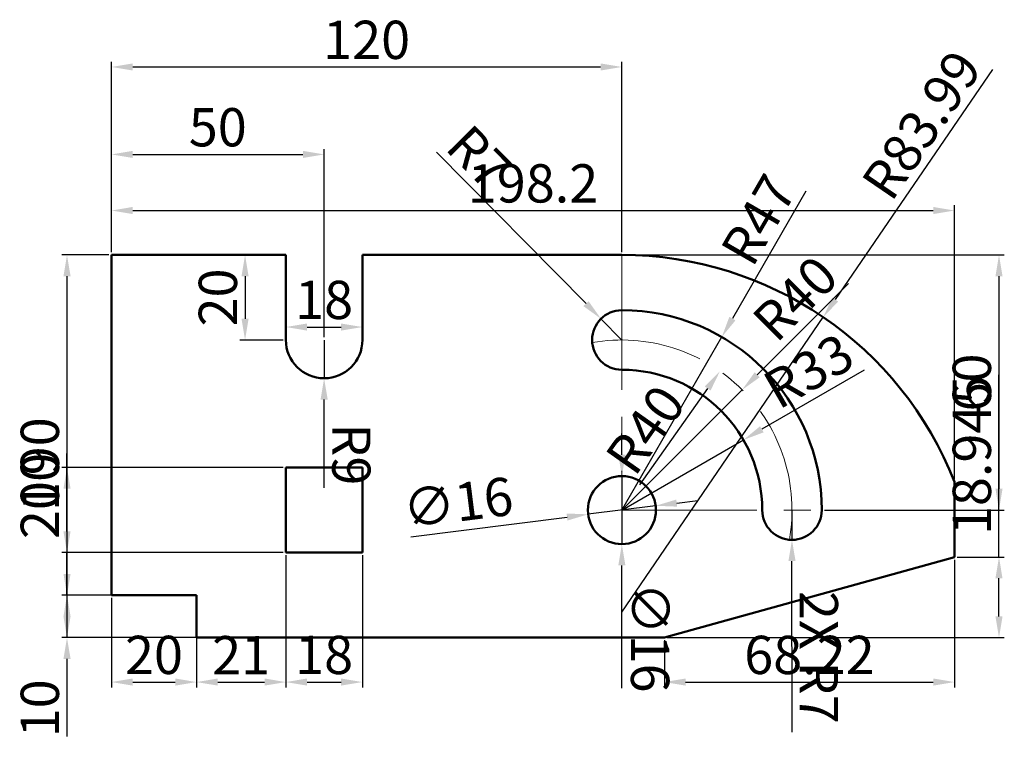
# Model space of a CAD drawing. Units: millimetres. Extents: x 2223 to 2454, y 1457 to 1626.
import ezdxf

# ---------------------------------------------------------------- set-up
doc = ezdxf.new("R2010")
doc.units = ezdxf.units.MM
doc.linetypes.add('CENTER', pattern=[50.8, 31.75, -6.35, 6.35, -6.35])
for name, color, linetype, lineweight in [('M-CNTR', 4, 'CENTER', 18), ('M-DIMS', 2, 'Continuous', 25), ('M-OUTL', 7, 'Continuous', 50)]:
    doc.layers.add(name, color=color, linetype=linetype, lineweight=lineweight)
doc.styles.get("Standard").update_dxf_attribs({"font": 'arial.ttf'})
doc.dimstyles.new('ISO-25', dxfattribs={"dimtxt": 9, "dimasz": 5, "dimexe": 1.25, "dimexo": 0.625, "dimtad": 1, "dimtxsty": 'Standard', "dimcen": 2.5, "dimadec": 0, "dimazin": 0, "dimtfac": 1, "dimtmove": 0, "dimatfit": 3, "dimfxl": 1, "dimarcsym": 0})

# ---------------------------------------------------------------- blocks, each defined once
blk = doc.blocks.new('*D1')
at = {"layer": 'Defpoints', "color": 0, "transparency": 16777216}
for p in [(2294.23, 1594.38), (2244.23, 1570.73), (2294.23, 1550.73)]:
    blk.add_point(p, dxfattribs=at)
at = {"layer": 'M-DIMS', "color": 0, "lineweight": -2, "transparency": 16777216}
for p, q in [((2244.23, 1571.36), (2244.23, 1595.63)), ((2294.23, 1551.36), (2294.23, 1595.63)), ((2249.23, 1594.38), (2289.23, 1594.38))]:
    blk.add_line(p, q, dxfattribs=at)
at = {"layer": 'M-DIMS', "color": 0, "transparency": 16777216}
for points in [[(2249.23, 1595.21), (2249.23, 1593.54), (2244.23, 1594.38)], [(2289.23, 1595.21), (2289.23, 1593.54), (2294.23, 1594.38)]]:
    blk.add_solid(points, dxfattribs=at)
at = {"layer": 'M-DIMS', "color": 0, "transparency": 16777216, "insert": (2269.23, 1599.6), "char_height": 9, "attachment_point": 5}
blk.add_mtext('50', dxfattribs=at)
blk = doc.blocks.new('*D2')
at = {"layer": 'Defpoints', "color": 0, "transparency": 16777216}
for p in [(2364.23, 1614.94), (2244.23, 1570.73), (2364.23, 1570.73)]:
    blk.add_point(p, dxfattribs=at)
at = {"layer": 'M-DIMS', "color": 0, "lineweight": -2, "transparency": 16777216}
for p, q in [((2244.23, 1571.36), (2244.23, 1616.19)), ((2364.23, 1571.36), (2364.23, 1616.19)), ((2249.23, 1614.94), (2359.23, 1614.94))]:
    blk.add_line(p, q, dxfattribs=at)
at = {"layer": 'M-DIMS', "color": 0, "transparency": 16777216}
for points in [[(2249.23, 1615.77), (2249.23, 1614.11), (2244.23, 1614.94)], [(2359.23, 1615.77), (2359.23, 1614.11), (2364.23, 1614.94)]]:
    blk.add_solid(points, dxfattribs=at)
at = {"layer": 'M-DIMS', "color": 0, "transparency": 16777216, "insert": (2304.23, 1620.16), "char_height": 9, "attachment_point": 5}
blk.add_mtext('120', dxfattribs=at)
blk = doc.blocks.new('*D3')
at = {"layer": 'Defpoints', "color": 0, "transparency": 16777216}
for p in [(2285.23, 1570.73), (2303.23, 1570.73), (2303.23, 1553.78)]:
    blk.add_point(p, dxfattribs=at)
at = {"layer": 'M-DIMS', "color": 0, "lineweight": -2, "transparency": 16777216}
for p, q in [((2285.23, 1570.11), (2285.23, 1552.53)), ((2303.23, 1570.11), (2303.23, 1552.53)), ((2290.23, 1553.78), (2298.23, 1553.78))]:
    blk.add_line(p, q, dxfattribs=at)
at = {"layer": 'M-DIMS', "color": 0, "transparency": 16777216}
for points in [[(2290.23, 1554.61), (2290.23, 1552.94), (2285.23, 1553.78)], [(2298.23, 1554.61), (2298.23, 1552.94), (2303.23, 1553.78)]]:
    blk.add_solid(points, dxfattribs=at)
at = {"layer": 'M-DIMS', "color": 0, "transparency": 16777216, "insert": (2294.23, 1559), "char_height": 9, "attachment_point": 5}
blk.add_mtext('18', dxfattribs=at)
blk = doc.blocks.new('*D4')
at = {"layer": 'Defpoints', "color": 0, "transparency": 16777216}
for p in [(2285.23, 1570.73), (2275.64, 1550.73), (2285.23, 1550.73)]:
    blk.add_point(p, dxfattribs=at)
at = {"layer": 'M-DIMS', "color": 0, "lineweight": -2, "transparency": 16777216}
for p, q in [((2284.61, 1570.73), (2274.39, 1570.73)), ((2275.64, 1565.73), (2275.64, 1555.73)), ((2284.61, 1550.73), (2274.39, 1550.73))]:
    blk.add_line(p, q, dxfattribs=at)
at = {"layer": 'M-DIMS', "color": 0, "transparency": 16777216}
for points in [[(2274.81, 1565.73), (2276.47, 1565.73), (2275.64, 1570.73)], [(2274.81, 1555.73), (2276.47, 1555.73), (2275.64, 1550.73)]]:
    blk.add_solid(points, dxfattribs=at)
at = {"layer": 'M-DIMS', "color": 0, "transparency": 16777216, "insert": (2270.42, 1560.73), "char_height": 9, "attachment_point": 5, "rotation": 90}
blk.add_mtext('20', dxfattribs=at)
blk = doc.blocks.new('*D5')
at = {"layer": 'Defpoints', "color": 0, "transparency": 16777216}
for p in [(2359.32, 1555.72), (2364.23, 1550.73)]:
    blk.add_point(p, dxfattribs=at)
at = {"layer": 'M-DIMS', "color": 0, "lineweight": -2, "transparency": 16777216}
for p, q in [((2320.69, 1594.87), (2355.81, 1559.28)), ((2364.23, 1550.73), (2359.32, 1555.72))]:
    blk.add_line(p, q, dxfattribs=at)
at = {"layer": 'M-DIMS', "color": 0, "transparency": 16777216}
blk.add_solid([(2356.4, 1559.86), (2355.21, 1558.69), (2359.32, 1555.72)], dxfattribs=at)
at = {"layer": 'M-DIMS', "color": 0, "transparency": 16777216, "insert": (2329.87, 1592.86), "char_height": 9, "attachment_point": 5, "rotation": 314.6114}
blk.add_mtext('R7', dxfattribs=at)
blk = doc.blocks.new('*D6')
at = {"layer": 'Defpoints', "color": 0, "transparency": 16777216}
for p in [(2387.3, 1543.42), (2364.23, 1510.73)]:
    blk.add_point(p, dxfattribs=at)
at = {"layer": 'M-DIMS', "color": 0, "lineweight": -2, "transparency": 16777216}
blk.add_line((2368.43, 1516.68), (2384.41, 1539.33), dxfattribs=at)
at = {"layer": 'M-DIMS', "color": 0, "transparency": 16777216}
blk.add_solid([(2383.73, 1539.81), (2385.09, 1538.85), (2387.3, 1543.42)], dxfattribs=at)
at = {"layer": 'M-DIMS', "color": 0, "transparency": 16777216, "insert": (2370.71, 1528.97), "char_height": 9, "attachment_point": 5, "rotation": 54.7921}
blk.add_mtext('R40', dxfattribs=at)
blk = doc.blocks.new('*D7')
at = {"layer": 'Defpoints', "color": 0, "transparency": 16777216}
for p in [(2372.17, 1511.74), (2356.3, 1509.73)]:
    blk.add_point(p, dxfattribs=at)
at = {"layer": 'M-DIMS', "color": 0, "lineweight": -2, "transparency": 16777216}
for p, q in [((2372.17, 1511.74), (2356.3, 1509.73)), ((2377.13, 1512.37), (2382.09, 1513)), ((2314.65, 1504.44), (2351.34, 1509.1))]:
    blk.add_line(p, q, dxfattribs=at)
at = {"layer": 'M-DIMS', "color": 0, "transparency": 16777216}
for points in [[(2377.03, 1513.2), (2377.24, 1511.54), (2372.17, 1511.74)], [(2351.23, 1509.92), (2351.44, 1508.27), (2356.3, 1509.73)]]:
    blk.add_solid(points, dxfattribs=at)
at = {"layer": 'M-DIMS', "color": 0, "transparency": 16777216, "insert": (2325.83, 1511.38), "char_height": 9, "attachment_point": 5, "rotation": 7.2276}
blk.add_mtext('∅16', dxfattribs=at)
blk = doc.blocks.new('*D8')
at = {"layer": 'Defpoints', "color": 0, "transparency": 16777216}
for p in [(2442.45, 1581.18), (2244.23, 1570.73), (2442.45, 1517.34)]:
    blk.add_point(p, dxfattribs=at)
at = {"layer": 'M-DIMS', "color": 0, "lineweight": -2, "transparency": 16777216}
for p, q in [((2244.23, 1571.36), (2244.23, 1582.43)), ((2249.23, 1581.18), (2437.45, 1581.18)), ((2442.45, 1517.97), (2442.45, 1582.43))]:
    blk.add_line(p, q, dxfattribs=at)
at = {"layer": 'M-DIMS', "color": 0, "transparency": 16777216}
for points in [[(2249.23, 1582.02), (2249.23, 1580.35), (2244.23, 1581.18)], [(2437.45, 1582.02), (2437.45, 1580.35), (2442.45, 1581.18)]]:
    blk.add_solid(points, dxfattribs=at)
at = {"layer": 'M-DIMS', "color": 0, "transparency": 16777216, "insert": (2343.34, 1586.4), "char_height": 9, "attachment_point": 5}
blk.add_mtext('198.2', dxfattribs=at)
blk = doc.blocks.new('*D9')
at = {"layer": 'Defpoints', "color": 0, "transparency": 16777216}
for p in [(2244.23, 1570.73), (2233.78, 1480.73), (2374.23, 1480.73)]:
    blk.add_point(p, dxfattribs=at)
at = {"layer": 'M-DIMS', "color": 0, "lineweight": -2, "transparency": 16777216}
for p, q in [((2243.61, 1570.73), (2232.53, 1570.73)), ((2233.78, 1565.73), (2233.78, 1485.73)), ((2373.61, 1480.73), (2232.53, 1480.73))]:
    blk.add_line(p, q, dxfattribs=at)
at = {"layer": 'M-DIMS', "color": 0, "transparency": 16777216}
for points in [[(2232.95, 1565.73), (2234.62, 1565.73), (2233.78, 1570.73)], [(2232.95, 1485.73), (2234.62, 1485.73), (2233.78, 1480.73)]]:
    blk.add_solid(points, dxfattribs=at)
at = {"layer": 'M-DIMS', "color": 0, "transparency": 16777216, "insert": (2228.56, 1525.73), "char_height": 9, "attachment_point": 5, "rotation": 90}
blk.add_mtext('90', dxfattribs=at)
blk = doc.blocks.new('*D10')
at = {"layer": 'Defpoints', "color": 0, "transparency": 16777216}
for p in [(2244.23, 1490.73), (2264.23, 1490.73), (2264.23, 1470.28)]:
    blk.add_point(p, dxfattribs=at)
at = {"layer": 'M-DIMS', "color": 0, "lineweight": -2, "transparency": 16777216}
for p, q in [((2244.23, 1490.11), (2244.23, 1469.03)), ((2264.23, 1490.11), (2264.23, 1469.03)), ((2249.23, 1470.28), (2259.23, 1470.28))]:
    blk.add_line(p, q, dxfattribs=at)
at = {"layer": 'M-DIMS', "color": 0, "transparency": 16777216}
for points in [[(2249.23, 1471.12), (2249.23, 1469.45), (2244.23, 1470.28)], [(2259.23, 1471.12), (2259.23, 1469.45), (2264.23, 1470.28)]]:
    blk.add_solid(points, dxfattribs=at)
at = {"layer": 'M-DIMS', "color": 0, "transparency": 16777216, "insert": (2254.23, 1475.5), "char_height": 9, "attachment_point": 5}
blk.add_mtext('20', dxfattribs=at)
blk = doc.blocks.new('*D11')
at = {"layer": 'Defpoints', "color": 0, "transparency": 16777216}
for p in [(2264.23, 1490.73), (2233.78, 1480.73), (2264.23, 1480.73)]:
    blk.add_point(p, dxfattribs=at)
at = {"layer": 'M-DIMS', "color": 0, "lineweight": -2, "transparency": 16777216}
for p, q in [((2233.78, 1495.73), (2233.78, 1500.73)), ((2263.61, 1490.73), (2232.53, 1490.73)), ((2233.78, 1490.73), (2233.78, 1480.73)), ((2263.61, 1480.73), (2232.53, 1480.73)), ((2233.78, 1475.73), (2233.78, 1457.47))]:
    blk.add_line(p, q, dxfattribs=at)
at = {"layer": 'M-DIMS', "color": 0, "transparency": 16777216}
for points in [[(2232.95, 1495.73), (2234.62, 1495.73), (2233.78, 1490.73)], [(2232.95, 1475.73), (2234.62, 1475.73), (2233.78, 1480.73)]]:
    blk.add_solid(points, dxfattribs=at)
at = {"layer": 'M-DIMS', "color": 0, "transparency": 16777216, "insert": (2228.56, 1464.1), "char_height": 9, "attachment_point": 5, "rotation": 90}
blk.add_mtext('10', dxfattribs=at)
blk = doc.blocks.new('*D12')
at = {"layer": 'Defpoints', "color": 0, "transparency": 16777216}
for p in [(2442.45, 1499.68), (2374.23, 1480.73), (2442.45, 1470.28)]:
    blk.add_point(p, dxfattribs=at)
at = {"layer": 'M-DIMS', "color": 0, "lineweight": -2, "transparency": 16777216}
for p, q in [((2442.45, 1499.05), (2442.45, 1469.03)), ((2374.23, 1480.11), (2374.23, 1469.03)), ((2379.23, 1470.28), (2437.45, 1470.28))]:
    blk.add_line(p, q, dxfattribs=at)
at = {"layer": 'M-DIMS', "color": 0, "transparency": 16777216}
for points in [[(2379.23, 1471.12), (2379.23, 1469.45), (2374.23, 1470.28)], [(2437.45, 1471.12), (2437.45, 1469.45), (2442.45, 1470.28)]]:
    blk.add_solid(points, dxfattribs=at)
at = {"layer": 'M-DIMS', "color": 0, "transparency": 16777216, "insert": (2408.34, 1475.5), "char_height": 9, "attachment_point": 5}
blk.add_mtext('68.22', dxfattribs=at)
blk = doc.blocks.new('*D13')
at = {"layer": 'Defpoints', "color": 0, "transparency": 16777216}
for p in [(2442.45, 1499.68), (2452.9, 1499.68), (2374.23, 1480.73)]:
    blk.add_point(p, dxfattribs=at)
at = {"layer": 'M-DIMS', "color": 0, "lineweight": -2, "transparency": 16777216}
for p, q in [((2452.9, 1499.68), (2452.9, 1542.51)), ((2443.08, 1499.68), (2454.15, 1499.68)), ((2452.9, 1485.73), (2452.9, 1494.68)), ((2374.86, 1480.73), (2454.15, 1480.73))]:
    blk.add_line(p, q, dxfattribs=at)
at = {"layer": 'M-DIMS', "color": 0, "transparency": 16777216}
for points in [[(2452.07, 1494.68), (2453.73, 1494.68), (2452.9, 1499.68)], [(2452.07, 1485.73), (2453.73, 1485.73), (2452.9, 1480.73)]]:
    blk.add_solid(points, dxfattribs=at)
at = {"layer": 'M-DIMS', "color": 0, "transparency": 16777216, "insert": (2447.68, 1523.6), "char_height": 9, "attachment_point": 5, "rotation": 90}
blk.add_mtext('18.945', dxfattribs=at)
blk = doc.blocks.new('*D14')
at = {"layer": 'Defpoints', "color": 0, "transparency": 16777216}
for p in [(2285.23, 1500.73), (2303.23, 1500.73), (2303.23, 1470.28)]:
    blk.add_point(p, dxfattribs=at)
at = {"layer": 'M-DIMS', "color": 0, "lineweight": -2, "transparency": 16777216}
for p, q in [((2285.23, 1500.11), (2285.23, 1469.03)), ((2303.23, 1500.11), (2303.23, 1469.03)), ((2290.23, 1470.28), (2298.23, 1470.28))]:
    blk.add_line(p, q, dxfattribs=at)
at = {"layer": 'M-DIMS', "color": 0, "transparency": 16777216}
for points in [[(2290.23, 1471.12), (2290.23, 1469.45), (2285.23, 1470.28)], [(2298.23, 1471.12), (2298.23, 1469.45), (2303.23, 1470.28)]]:
    blk.add_solid(points, dxfattribs=at)
at = {"layer": 'M-DIMS', "color": 0, "transparency": 16777216, "insert": (2294.23, 1475.5), "char_height": 9, "attachment_point": 5}
blk.add_mtext('18', dxfattribs=at)
blk = doc.blocks.new('*D15')
at = {"layer": 'Defpoints', "color": 0, "transparency": 16777216}
for p in [(2233.78, 1520.73), (2285.23, 1520.73), (2285.23, 1500.73)]:
    blk.add_point(p, dxfattribs=at)
at = {"layer": 'M-DIMS', "color": 0, "lineweight": -2, "transparency": 16777216}
for p, q in [((2284.61, 1520.73), (2232.53, 1520.73)), ((2233.78, 1505.73), (2233.78, 1515.73)), ((2284.61, 1500.73), (2232.53, 1500.73))]:
    blk.add_line(p, q, dxfattribs=at)
at = {"layer": 'M-DIMS', "color": 0, "transparency": 16777216}
for points in [[(2232.95, 1515.73), (2234.62, 1515.73), (2233.78, 1520.73)], [(2232.95, 1505.73), (2234.62, 1505.73), (2233.78, 1500.73)]]:
    blk.add_solid(points, dxfattribs=at)
at = {"layer": 'M-DIMS', "color": 0, "transparency": 16777216, "insert": (2228.56, 1510.73), "char_height": 9, "attachment_point": 5, "rotation": 90}
blk.add_mtext('20', dxfattribs=at)
blk = doc.blocks.new('*D16')
at = {"layer": 'Defpoints', "color": 0, "transparency": 16777216}
for p in [(2285.23, 1500.73), (2264.23, 1480.73), (2285.23, 1470.28)]:
    blk.add_point(p, dxfattribs=at)
at = {"layer": 'M-DIMS', "color": 0, "lineweight": -2, "transparency": 16777216}
for p, q in [((2285.23, 1500.11), (2285.23, 1469.03)), ((2264.23, 1480.11), (2264.23, 1469.03)), ((2269.23, 1470.28), (2280.23, 1470.28))]:
    blk.add_line(p, q, dxfattribs=at)
at = {"layer": 'M-DIMS', "color": 0, "transparency": 16777216}
for points in [[(2269.23, 1471.12), (2269.23, 1469.45), (2264.23, 1470.28)], [(2280.23, 1471.12), (2280.23, 1469.45), (2285.23, 1470.28)]]:
    blk.add_solid(points, dxfattribs=at)
at = {"layer": 'M-DIMS', "color": 0, "transparency": 16777216, "insert": (2274.73, 1475.43), "char_height": 9, "attachment_point": 5}
blk.add_mtext('21', dxfattribs=at)
blk = doc.blocks.new('*D17')
at = {"layer": 'Defpoints', "color": 0, "transparency": 16777216}
for p in [(2233.78, 1500.73), (2285.23, 1500.73), (2264.23, 1490.73)]:
    blk.add_point(p, dxfattribs=at)
at = {"layer": 'M-DIMS', "color": 0, "lineweight": -2, "transparency": 16777216}
for p, q in [((2233.78, 1505.73), (2233.78, 1524)), ((2284.61, 1500.73), (2232.53, 1500.73)), ((2233.78, 1490.73), (2233.78, 1500.73)), ((2263.61, 1490.73), (2232.53, 1490.73)), ((2233.78, 1485.73), (2233.78, 1480.73))]:
    blk.add_line(p, q, dxfattribs=at)
at = {"layer": 'M-DIMS', "color": 0, "transparency": 16777216}
for points in [[(2232.95, 1505.73), (2234.62, 1505.73), (2233.78, 1500.73)], [(2232.95, 1485.73), (2234.62, 1485.73), (2233.78, 1490.73)]]:
    blk.add_solid(points, dxfattribs=at)
at = {"layer": 'M-DIMS', "color": 0, "transparency": 16777216, "insert": (2228.56, 1517.37), "char_height": 9, "attachment_point": 5, "rotation": 90}
blk.add_mtext('10', dxfattribs=at)
blk = doc.blocks.new('*D18')
at = {"layer": 'Defpoints', "color": 0, "transparency": 16777216}
for p in [(2364.23, 1570.73), (2411.23, 1510.73), (2452.9, 1510.73)]:
    blk.add_point(p, dxfattribs=at)
at = {"layer": 'M-DIMS', "color": 0, "lineweight": -2, "transparency": 16777216}
for p, q in [((2364.86, 1570.73), (2454.15, 1570.73)), ((2452.9, 1565.73), (2452.9, 1515.73)), ((2411.86, 1510.73), (2454.15, 1510.73))]:
    blk.add_line(p, q, dxfattribs=at)
at = {"layer": 'M-DIMS', "color": 0, "transparency": 16777216}
for points in [[(2452.07, 1565.73), (2453.73, 1565.73), (2452.9, 1570.73)], [(2452.07, 1515.73), (2453.73, 1515.73), (2452.9, 1510.73)]]:
    blk.add_solid(points, dxfattribs=at)
at = {"layer": 'M-DIMS', "color": 0, "transparency": 16777216, "insert": (2447.68, 1540.73), "char_height": 9, "attachment_point": 5, "rotation": 90}
blk.add_mtext('60', dxfattribs=at)
blk = doc.blocks.new('*D19')
at = {"layer": 'Defpoints', "color": 0, "transparency": 16777216}
for p in [(2411.58, 1556.11), (2364.23, 1486.75)]:
    blk.add_point(p, dxfattribs=at)
at = {"layer": 'M-DIMS', "color": 0, "lineweight": -2, "transparency": 16777216}
for p, q in [((2451.34, 1614.36), (2414.4, 1560.24)), ((2364.23, 1486.75), (2411.58, 1556.11))]:
    blk.add_line(p, q, dxfattribs=at)
at = {"layer": 'M-DIMS', "color": 0, "transparency": 16777216}
blk.add_solid([(2413.72, 1560.71), (2415.09, 1559.77), (2411.58, 1556.11)], dxfattribs=at)
at = {"layer": 'M-DIMS', "color": 0, "transparency": 16777216, "insert": (2435.68, 1600.68), "char_height": 9, "attachment_point": 5, "rotation": 55.6818}
blk.add_mtext('R83.99', dxfattribs=at)
blk = doc.blocks.new('*D20')
at = {"layer": 'Defpoints', "color": 0, "transparency": 16777216}
for p in [(2387.73, 1551.44), (2364.23, 1510.73)]:
    blk.add_point(p, dxfattribs=at)
at = {"layer": 'M-DIMS', "color": 0, "lineweight": -2, "transparency": 16777216}
for p, q in [((2407.51, 1585.72), (2390.23, 1555.77)), ((2364.23, 1510.73), (2387.73, 1551.44))]:
    blk.add_line(p, q, dxfattribs=at)
at = {"layer": 'M-DIMS', "color": 0, "transparency": 16777216}
blk.add_solid([(2389.51, 1556.19), (2390.95, 1555.35), (2387.73, 1551.44)], dxfattribs=at)
at = {"layer": 'M-DIMS', "color": 0, "transparency": 16777216, "insert": (2397.39, 1578.42), "char_height": 9, "attachment_point": 5, "rotation": 60.0058}
blk.add_mtext('R47', dxfattribs=at)
blk = doc.blocks.new('*D21')
at = {"layer": 'Defpoints', "color": 0, "transparency": 16777216}
for p in [(2392.52, 1539.02), (2364.23, 1510.73)]:
    blk.add_point(p, dxfattribs=at)
at = {"layer": 'M-DIMS', "color": 0, "lineweight": -2, "transparency": 16777216}
for p, q in [((2417.52, 1564.02), (2396.05, 1542.55)), ((2364.23, 1510.73), (2392.52, 1539.02))]:
    blk.add_line(p, q, dxfattribs=at)
at = {"layer": 'M-DIMS', "color": 0, "transparency": 16777216}
blk.add_solid([(2395.46, 1543.14), (2396.64, 1541.96), (2392.52, 1539.02)], dxfattribs=at)
at = {"layer": 'M-DIMS', "color": 0, "transparency": 16777216, "insert": (2405.8, 1559.68), "char_height": 9, "attachment_point": 5, "rotation": 45.0002}
blk.add_mtext('R40', dxfattribs=at)
blk = doc.blocks.new('*D22')
at = {"layer": 'Defpoints', "color": 0, "transparency": 16777216}
for p in [(2392.81, 1527.23), (2364.23, 1510.73)]:
    blk.add_point(p, dxfattribs=at)
at = {"layer": 'M-DIMS', "color": 0, "lineweight": -2, "transparency": 16777216}
for p, q in [((2421.18, 1543.61), (2397.14, 1529.73)), ((2364.23, 1510.73), (2392.81, 1527.23))]:
    blk.add_line(p, q, dxfattribs=at)
at = {"layer": 'M-DIMS', "color": 0, "transparency": 16777216}
blk.add_solid([(2396.73, 1530.45), (2397.56, 1529.01), (2392.81, 1527.23)], dxfattribs=at)
at = {"layer": 'M-DIMS', "color": 0, "transparency": 16777216, "insert": (2408.72, 1542.44), "char_height": 9, "attachment_point": 5, "rotation": 29.997}
blk.add_mtext('R33', dxfattribs=at)
blk = doc.blocks.new('*D23')
at = {"layer": 'Defpoints', "color": 0, "transparency": 16777216}
for p in [(2294.23, 1550.73), (2294.23, 1541.73)]:
    blk.add_point(p, dxfattribs=at)
at = {"layer": 'M-DIMS', "color": 0, "lineweight": -2, "transparency": 16777216}
for p, q in [((2294.23, 1550.73), (2294.23, 1541.73)), ((2294.24, 1515.95), (2294.23, 1536.73))]:
    blk.add_line(p, q, dxfattribs=at)
at = {"layer": 'M-DIMS', "color": 0, "transparency": 16777216}
blk.add_solid([(2295.07, 1536.73), (2293.4, 1536.73), (2294.23, 1541.73)], dxfattribs=at)
at = {"layer": 'M-DIMS', "color": 0, "transparency": 16777216, "insert": (2299.46, 1523.84), "char_height": 9, "attachment_point": 5, "rotation": 270.0028}
blk.add_mtext('R9', dxfattribs=at)
blk = doc.blocks.new('*D24')
at = {"layer": 'Defpoints', "color": 0, "transparency": 16777216}
for p in [(2364.23, 1518.73), (2364.23, 1502.73)]:
    blk.add_point(p, dxfattribs=at)
at = {"layer": 'M-DIMS', "color": 0, "lineweight": -2, "transparency": 16777216}
for p, q in [((2364.23, 1523.73), (2364.23, 1528.73)), ((2364.23, 1518.73), (2364.23, 1502.73)), ((2364.24, 1468.81), (2364.23, 1497.73))]:
    blk.add_line(p, q, dxfattribs=at)
at = {"layer": 'M-DIMS', "color": 0, "transparency": 16777216}
for points in [[(2365.07, 1523.73), (2363.4, 1523.73), (2364.23, 1518.73)], [(2365.07, 1497.73), (2363.4, 1497.73), (2364.23, 1502.73)]]:
    blk.add_solid(points, dxfattribs=at)
at = {"layer": 'M-DIMS', "color": 0, "transparency": 16777216, "insert": (2369.71, 1480.77), "char_height": 9, "attachment_point": 5, "rotation": 270.0031}
blk.add_mtext('∅16', dxfattribs=at)
blk = doc.blocks.new('*D25')
at = {"layer": 'Defpoints', "color": 0, "transparency": 16777216}
for p in [(2404.23, 1510.73), (2404.23, 1503.73)]:
    blk.add_point(p, dxfattribs=at)
at = {"layer": 'M-DIMS', "color": 0, "lineweight": -2, "transparency": 16777216}
for p, q in [((2404.23, 1510.73), (2404.23, 1503.73)), ((2404.24, 1458.48), (2404.23, 1498.73))]:
    blk.add_line(p, q, dxfattribs=at)
at = {"layer": 'M-DIMS', "color": 0, "transparency": 16777216}
blk.add_solid([(2405.07, 1498.73), (2403.4, 1498.73), (2404.23, 1503.73)], dxfattribs=at)
at = {"layer": 'M-DIMS', "color": 0, "transparency": 16777216, "insert": (2409.38, 1476.11), "char_height": 9, "attachment_point": 5, "rotation": 270.0036}
blk.add_mtext('2X R7', dxfattribs=at)

msp = doc.modelspace()

# ---------------------------------------------------------------- linework, layer by layer
at = {"layer": 'M-CNTR'}
for p, q in [((2364.2336, 1570.7334), (2364.2336, 1510.7334)), ((2364.2336, 1510.7334), (2419.4078, 1510.7334))]:
    msp.add_line(p, q, dxfattribs=at)
msp.add_arc((2364.2336, 1510.7334), 40, 349.9604, 100.0396, dxfattribs=at)
at = {"layer": 'M-OUTL'}
for p, q in [((2244.2336, 1570.7334), (2285.2336, 1570.7334)), ((2244.2336, 1570.7334), (2285.2336, 1570.7334)), ((2244.2336, 1570.7334), (2244.2336, 1490.7334)), ((2285.2336, 1550.7334), (2285.2336, 1570.7334)), ((2303.2336, 1570.7334), (2364.2336, 1570.7334)), ((2303.2336, 1570.7334), (2303.2336, 1550.7334)), ((2294.2336, 1520.7334), (2285.2336, 1520.7334)), ((2285.2336, 1500.7334), (2285.2336, 1520.7334)), ((2294.2336, 1520.7334), (2303.2336, 1520.7334)), ((2303.2336, 1520.7334), (2303.2336, 1500.7334)), ((2442.4504, 1517.3406), (2442.4504, 1499.6789)), ((2303.2336, 1500.7334), (2285.2336, 1500.7334)), ((2374.2336, 1480.7334), (2442.4504, 1499.6789)), ((2244.2336, 1490.7334), (2264.2336, 1490.7334)), ((2264.2336, 1490.7334), (2264.2336, 1480.7334)), ((2264.2336, 1480.7334), (2324.2336, 1480.7334)), ((2324.2336, 1480.7334), (2374.2336, 1480.7334))]:
    msp.add_line(p, q, dxfattribs=at)
msp.add_circle((2364.2336, 1510.7334), 8, dxfattribs=at)
for centre, radius, start, end in [((2364.2336, 1486.7458), 83.9876, 21.363165, 90), ((2364.2336, 1550.7334), 7, 90, 270), ((2364.2336, 1510.7334), 47, 0, 90), ((2294.2336, 1550.7334), 9, 180, 0), ((2364.2336, 1510.7334), 33, 0, 90), ((2404.2336, 1510.7334), 7, 180, 0)]:
    msp.add_arc(centre, radius, start, end, dxfattribs=at)

# ---------------------------------------------------------------- dimensions: what is measured, and where the dimension line sits
at = {"layer": 'M-DIMS'}
for base, p1, p2, override, picture, middle in [((2364.2336, 1614.9388), (2244.2336, 1570.7334), (2364.2336, 1570.7334), {"dimclrd": 0, "dimclre": 0, "dimclrt": 0}, '*D2', (2304.2336, 1620.159)), ((2294.2336, 1594.3771), (2244.2336, 1570.7334), (2294.2336, 1550.7334), {"dimclrd": 0, "dimclre": 0, "dimclrt": 0}, '*D1', (2269.2336, 1599.5972)), ((2442.4504, 1581.1834), (2244.2336, 1570.7334), (2442.4504, 1517.3406), {"dimdec": 1, "dimlfac": 1, "dimrnd": 0, "dimzin": 0, "dimdsep": 46, "dimlunit": 2}, '*D8', (2343.342, 1586.4035)), ((2285.2336, 1470.2834), (2264.2336, 1480.7334), (2285.2336, 1500.7334), {"dimdec": 0, "dimlfac": 1, "dimrnd": 0, "dimzin": 0, "dimdsep": 46, "dimlunit": 2}, '*D16', (2274.7336, 1475.4268)), ((2303.2336, 1470.2834), (2285.2336, 1500.7334), (2303.2336, 1500.7334), {"dimdec": 0, "dimlfac": 1, "dimrnd": 0, "dimzin": 0, "dimdsep": 46, "dimlunit": 2}, '*D14', (2294.2336, 1475.5035)), ((2442.4504, 1470.2834), (2374.2336, 1480.7334), (2442.4504, 1499.6789), {"dimdec": 2, "dimlfac": 1, "dimrnd": 0, "dimzin": 0, "dimdsep": 46, "dimlunit": 2}, '*D12', (2408.342, 1475.5035)), ((2264.2336, 1470.2834), (2244.2336, 1490.7334), (2264.2336, 1490.7334), {"dimdec": 0, "dimlfac": 1, "dimrnd": 0, "dimzin": 0, "dimdsep": 46, "dimlunit": 2}, '*D10', (2254.2336, 1475.5035))]:
    dim = msp.add_linear_dim(base=base, p1=p1, p2=p2, dimstyle='ISO-25', override=override, dxfattribs=at)
    dim.commit()
    dim.dimension.update_dxf_attribs({"geometry": picture, "text_midpoint": middle})
for center, mpoint, override, picture, middle in [((2364.2336, 1486.7458), (2411.5848, 1556.1127), {"dimdec": 2, "dimlfac": 1, "dimrnd": 0, "dimzin": 0, "dimdsep": 46, "dimlunit": 2}, '*D19', (2439.9956, 1597.7329)), ((2364.2336, 1550.7334), (2359.3175, 1555.7166), {"dimclrd": 0, "dimclre": 0, "dimclrt": 0}, '*D5', (2326.222, 1589.264)), ((2364.2336, 1510.7334), (2387.7294, 1551.439), {"dimdec": 0, "dimlfac": 1, "dimrnd": 0, "dimzin": 0, "dimdsep": 46, "dimlunit": 2}, '*D20', (2401.8269, 1575.8623)), ((2364.2336, 1510.7334), (2392.5177, 1539.0177), {"dimdec": 0, "dimlfac": 1, "dimrnd": 0, "dimzin": 0, "dimdsep": 46, "dimlunit": 2}, '*D21', (2409.4883, 1555.9884)), ((2364.2336, 1510.7334), (2387.2953, 1543.416), {"dimclrd": 0, "dimclre": 0, "dimclrt": 0}, '*D6', (2374.979, 1525.9615))]:
    dim = msp.add_radius_dim(center=center, mpoint=mpoint, dimstyle='ISO-25', override=override, dxfattribs=at)
    dim.commit()
    dim.dimension.update_dxf_attribs({"geometry": picture, "text_midpoint": middle, "dimtype": 164})
for base, p1, p2, override, picture, middle in [((2233.7836, 1480.7334), (2244.2336, 1570.7334), (2374.2336, 1480.7334), {"dimdec": 0, "dimlfac": 1, "dimrnd": 0, "dimzin": 0, "dimdsep": 46, "dimlunit": 2}, '*D9', (2228.5634, 1525.7334)), ((2275.6416, 1550.7334), (2285.2336, 1570.7334), (2285.2336, 1550.7334), {"dimclrd": 0, "dimclre": 0, "dimclrt": 0}, '*D4', (2270.4215, 1560.7334)), ((2452.9004, 1510.7334), (2364.2336, 1570.7334), (2411.2336, 1510.7334), {"dimdec": 0, "dimlfac": 1, "dimrnd": 0, "dimzin": 0, "dimdsep": 46, "dimlunit": 2}, '*D18', (2447.6802, 1540.7334)), ((2452.90038, 1499.67885), (2374.23356, 1480.73339), (2442.45038, 1499.67885), {"dimdec": 3, "dimlfac": 1, "dimrnd": 0, "dimzin": 0, "dimdsep": 46, "dimlunit": 2}, '*D13', (2447.68022, 1523.59546)), ((2233.7836, 1500.7334), (2264.2336, 1490.7334), (2285.2336, 1500.7334), {"dimdec": 0, "dimlfac": 1, "dimrnd": 0, "dimzin": 0, "dimdsep": 46, "dimlunit": 2}, '*D17', (2228.5634, 1517.3655)), ((2233.7836, 1520.7334), (2285.2336, 1500.7334), (2285.2336, 1520.7334), {"dimdec": 0, "dimlfac": 1, "dimrnd": 0, "dimzin": 0, "dimdsep": 46, "dimlunit": 2}, '*D15', (2228.5634, 1510.7334)), ((2233.7836, 1480.7334), (2264.2336, 1490.7334), (2264.2336, 1480.7334), {"dimdec": 0, "dimlfac": 1, "dimrnd": 0, "dimzin": 0, "dimdsep": 46, "dimlunit": 2}, '*D11', (2228.5634, 1464.1012))]:
    dim = msp.add_linear_dim(base=base, p1=p1, p2=p2, angle=90, dimstyle='ISO-25', override=override, dxfattribs=at)
    dim.commit()
    dim.dimension.update_dxf_attribs({"geometry": picture, "text_midpoint": middle})
dim = msp.add_linear_dim(base=(2303.2336, 1553.7764), p1=(2285.2336, 1570.7334), p2=(2303.2336, 1570.7334), dimstyle='ISO-25', override={"dimclrd": 0, "dimclre": 0, "dimclrt": 0}, dxfattribs=at)
dim.commit()
dim.dimension.update_dxf_attribs({"geometry": '*D3', "text_midpoint": (2294.2336, 1553.7764), "dimtype": 160})
for center, mpoint, picture, middle in [((2364.2336, 1510.7334), (2392.8133, 1527.2319), '*D22', (2408.7161, 1542.4434)), ((2294.2336, 1550.7334), (2294.234, 1541.7334), '*D23', (2299.455, 1523.843))]:
    dim = msp.add_radius_dim(center=center, mpoint=mpoint, dimstyle='ISO-25', override={"dimdec": 0, "dimlfac": 1, "dimrnd": 0, "dimzin": 0, "dimdsep": 46, "dimlunit": 2}, dxfattribs=at)
    dim.commit()
    dim.dimension.update_dxf_attribs({"geometry": picture, "text_midpoint": middle})
dim = msp.add_diameter_dim_2p(p1=(2364.2331, 1518.7334), p2=(2364.234, 1502.7334), dimstyle='ISO-25', override={"dimdec": 0, "dimlfac": 1, "dimrnd": 0, "dimzin": 0, "dimdsep": 46, "dimlunit": 2}, dxfattribs=at)
dim.commit()
dim.dimension.update_dxf_attribs({"geometry": '*D24', "text_midpoint": (2364.2352, 1480.7694)})
dim = msp.add_diameter_dim_2p(p1=(2372.17, 1511.7399), p2=(2356.2971, 1509.7269), dimstyle='ISO-25', override={"dimclrd": 0, "dimclre": 0, "dimclrt": 0}, dxfattribs=at)
dim.commit()
dim.dimension.update_dxf_attribs({"geometry": '*D7', "text_midpoint": (2326.5151, 1505.95), "dimtype": 163})
dim = msp.add_radius_dim(center=(2404.2336, 1510.7334), mpoint=(2404.234, 1503.7334), text='2X <>', dimstyle='ISO-25', override={"dimdec": 0, "dimlfac": 1, "dimrnd": 0, "dimzin": 0, "dimdsep": 46, "dimlunit": 2}, dxfattribs=at)
dim.commit()
dim.dimension.update_dxf_attribs({"geometry": '*D25', "text_midpoint": (2409.3822, 1476.1063)})

doc.saveas('drawing.dxf')
